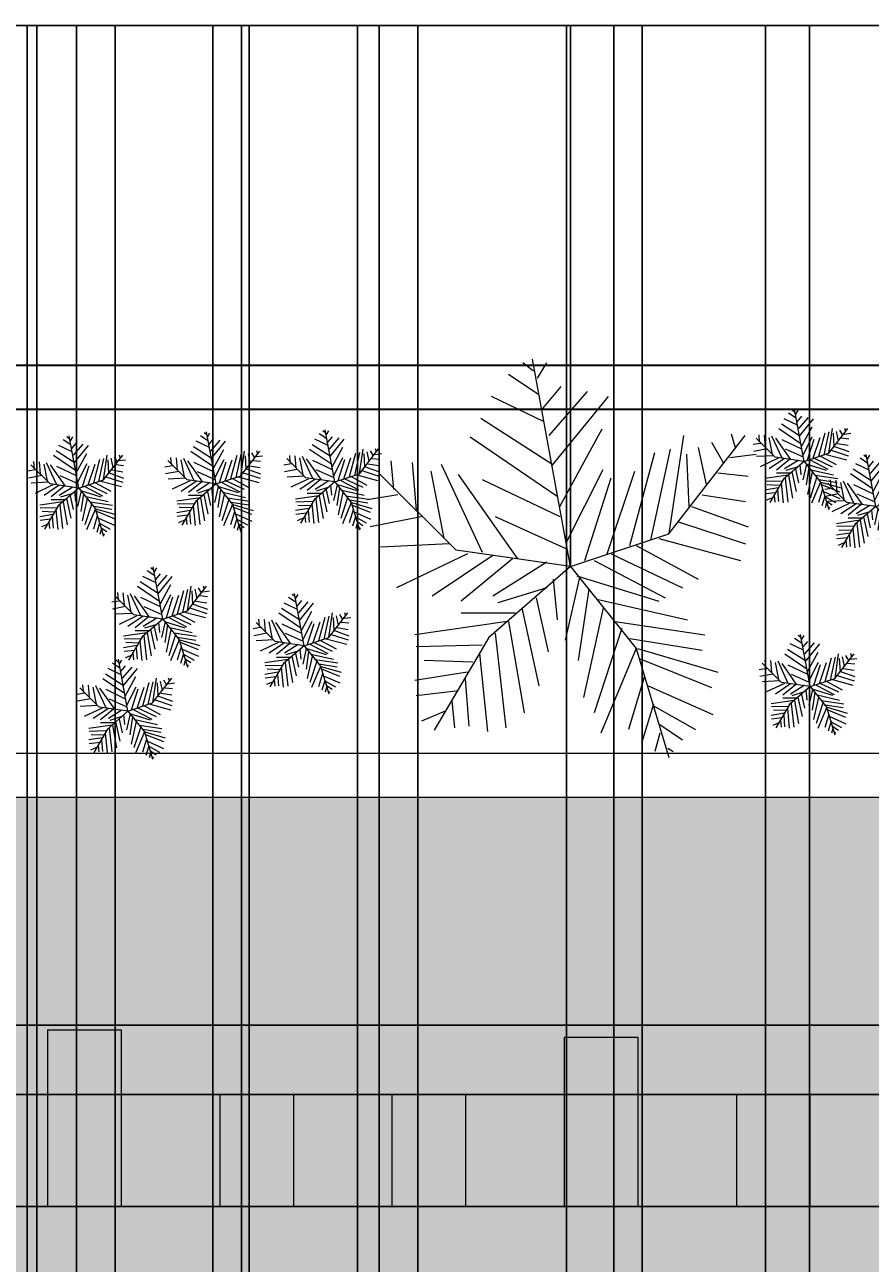
# Model space of a CAD drawing. Units: inches. Extents: x 818 to 1898, y 976 to 2364.
# Tile 94 of 96: x 1439 to 1612, y 2111 to 2364. Entities that reach past the tile are written whole.
import ezdxf

# ---------------------------------------------------------------- set-up
doc = ezdxf.new("R2010")
doc.units = ezdxf.units.IN
doc.header["$LTSCALE"] = 5
doc.header["$MEASUREMENT"] = 0
for name, color, linetype, lineweight in [('A-ANNO-DIMS', 2, 'Continuous', 18), ('C-PROP', 7, 'Continuous', 35), ('L-PAVE', 8, 'Continuous', 18), ('L-PLNT-BEDS', 94, 'Continuous', 18)]:
    doc.layers.add(name, color=color, linetype=linetype, lineweight=lineweight)
for name, color, linetype, lineweight, true_color in [('L-PAVE-PATT', 9, 'Continuous', 9, 0xc7c8ca), ('L-PLNT', 116, 'Continuous', 13, 0x136734), ('L-PLNT-PATT', 114, 'Continuous', 9, 0x139b48)]:
    doc.layers.add(name, color=color, linetype=linetype, lineweight=lineweight, true_color=true_color)
doc.styles.get("Standard").update_dxf_attribs({"font": 'arial.ttf'})
doc.dimstyles.get("Standard").update_dxf_attribs({"dimtxt": 0.18, "dimasz": 0.18, "dimexe": 0.18, "dimexo": 0.0625, "dimgap": 0.09, "dimtad": 0, "dimtih": 1, "dimtoh": 1, "dimdec": 4, "dimzin": 0, "dimdsep": 46, "dimtxsty": 'Standard', "dimcen": 0.09, "dimadec": 0, "dimazin": 0, "dimtfac": 1, "dimtdec": 4, "dimtofl": 0, "dimtmove": 0, "dimatfit": 3, "dimfxl": 1, "dimtolj": 1, "dimtzin": 0, "dimarcsym": 0})

# ---------------------------------------------------------------- blocks, each defined once
blk = doc.blocks.new('SHRUB-ACCENT')
for p, q in [((8.53, 19.84), (7.99, 20.28)), ((10.44, 9.82), (8.47, 20.47)), ((8.74, 19.5), (9.21, 20.28)), ((9.08, 17.24), (6.37, 18.54)), ((8.8, 18.63), (7.25, 19.67)), ((9.01, 17.93), (9.96, 19.06)), ((9.35, 16.54), (11.31, 18.8)), ((9.48, 14.98), (12.39, 18.54)), ((1.35, 13.77), (1.22, 15.24)), ((9.75, 13.42), (5.28, 16.46)), ((9.48, 15.07), (5.82, 17.41)), ((9.89, 12.9), (12.06, 16.89)), ((13.48, 10.9), (14.76, 15.68)), ((14.56, 11.16), (15.58, 15.85)), ((15.49, 11.5), (19.41, 16.55)), ((15.51, 11.51), (16.25, 16.54)), ((16.39, 15.59), (16.53, 12.9)), ((17, 15.94), (17.41, 14.03)), ((17.68, 16.2), (18.29, 15.16)), ((18.62, 15.42), (19.98, 15.59)), ((18.69, 16.63), (18.9, 15.94)), ((1.56, 13.51), (0, 13.25)), ((4.55, 10.66), (0.62, 14.58)), ((2.3, 15.16), (2.51, 12.72)), ((3.25, 14.72), (3.93, 11.25)), ((3.79, 15.07), (5.89, 10.55)), ((7.72, 10.21), (4.67, 14.55)), ((5.89, 14.29), (9.89, 12.38)), ((10.23, 11.07), (12.12, 14.81)), ((11.17, 10.12), (12.53, 14.37)), ((12.33, 10.47), (13.75, 14.72)), ((16.66, 12.9), (19.57, 11.86)), ((17.2, 13.51), (19.44, 13.16)), ((18.02, 14.63), (19.57, 14.46)), ((2.84, 12.38), (0.14, 11.86)), ((4.2, 10.99), (0.68, 10.81)), ((5.15, 10.47), (1.49, 8.73)), ((6.43, 10.38), (3.32, 8.3)), ((10.44, 9.82), (4.55, 10.66)), ((7.45, 10.21), (4.81, 8.04)), ((6.57, 12.38), (10.23, 10.73)), ((10.44, 9.82), (15.49, 11.5)), ((12.53, 10.47), (16.19, 8.73)), ((13.82, 10.9), (17, 9.16)), ((14.97, 11.25), (19.17, 10.12)), ((15.98, 12.12), (19.44, 10.99)), ((10.44, 9.82), (6.23, 6.17)), ((9.21, 10.03), (6.43, 8.3)), ((9.21, 8.73), (6.7, 7.95)), ((7.92, 7.69), (8.8, 3.69)), ((8.67, 8.21), (9.28, 5.43)), ((9.55, 9.16), (9.75, 7.08)), ((10.9, 9.25), (10.16, 6.04)), ((10.44, 9.82), (13.8, 5.61)), ((10.77, 9.34), (14.97, 8.04)), ((11.38, 8.64), (10.84, 5)), ((12.12, 7.69), (11.11, 3.09)), ((11.65, 10.12), (15.31, 8.21)), ((11.85, 8.12), (16.46, 7.08)), ((7.18, 6.99), (2.44, 6.3)), ((5.89, 5.78), (2.51, 5.69)), ((6.23, 6.17), (3.43, 1.4)), ((7.59, 7.43), (4.81, 7.43)), ((5.76, 5.34), (6.16, 1.35)), ((6.57, 6.39), (7.11, 1.52)), ((7.25, 6.99), (8.06, 2.31)), ((13.07, 6.65), (11.65, 2.31)), ((13.82, 5.6), (11.99, 1.26)), ((12.73, 6.99), (17.34, 6.3)), ((13.48, 6.13), (17.2, 5.52)), ((13.8, 5.61), (15.49, 0)), ((13.88, 5.6), (18.02, 4.39)), ((14.02, 5.08), (17.68, 3.61)), ((5.15, 4.39), (2.44, 3.95)), ((4.67, 3.43), (2.51, 3.17)), ((5.42, 4.91), (2.91, 5)), ((4.33, 2.91), (4.47, 1.52)), ((5.01, 4.04), (5.21, 1.61)), ((14.22, 4.13), (13.41, 1.44)), ((14.7, 2.74), (14.09, 0.74)), ((14.43, 3.69), (17.74, 2.22)), ((14.7, 2.65), (16.86, 1.44)), ((4, 2.39), (2.78, 1.87)), ((15.04, 1.26), (14.76, 0.31)), ((15.04, 1.7), (16.19, 0.92)), ((15.44, 0.48), (15.71, 0.31))]:
    blk.add_line(p, q)
blk = doc.blocks.new('PALM-BORDER')
for p, q in [((41.53, 39.05), (33.72, 81.45)), ((33.95, 78.95), (31.8, 80.68)), ((34.76, 77.57), (36.65, 80.68)), ((35.03, 74.11), (28.83, 78.26)), ((36.11, 68.59), (25.33, 73.77)), ((35.84, 71.35), (39.61, 75.84)), ((37.18, 65.82), (45, 74.8)), ((37.72, 59.6), (49.31, 73.77)), ((37.72, 59.95), (23.17, 69.28)), ((39.34, 51.31), (47.96, 67.2)), ((61.61, 45.75), (77.23, 65.83)), ((61.71, 45.79), (64.67, 65.82)), ((74.37, 66.17), (75.18, 63.4)), ((38.8, 53.39), (21.02, 65.48)), ((67.63, 63.4), (69.25, 55.81)), ((70.33, 64.44), (72.75, 60.3)), ((53.62, 43.37), (58.74, 62.37)), ((57.93, 44.41), (61.97, 63.06)), ((65.21, 62.02), (65.75, 51.31)), ((74.1, 61.33), (79.49, 62.02)), ((5.39, 54.77), (4.85, 60.64)), ((9.16, 60.3), (9.97, 50.62)), ((12.93, 58.57), (15.63, 44.75)), ((15.09, 59.95), (23.44, 41.99)), ((40.69, 44.06), (48.23, 58.91)), ((49.04, 41.64), (54.7, 58.57)), ((71.68, 58.22), (77.87, 57.53)), ((18.1, 42.4), (2.48, 58.02)), ((30.72, 40.61), (18.59, 57.88)), ((23.44, 56.84), (39.34, 49.24)), ((44.46, 40.26), (49.85, 57.19)), ((6.2, 53.73), (0, 52.7)), ((68.44, 53.73), (77.33, 52.35)), ((66.29, 51.31), (77.87, 47.17)), ((11.32, 49.24), (0.54, 47.17)), ((26.14, 49.24), (40.69, 42.68)), ((63.59, 48.21), (77.33, 43.71)), ((41.53, 39.05), (61.61, 45.75)), ((16.71, 43.71), (2.69, 43.02)), ((54.97, 43.37), (67.63, 36.46)), ((59.55, 44.75), (76.26, 40.26)), ((20.48, 41.64), (5.93, 34.73)), ((25.6, 41.3), (13.2, 33.01)), ((41.53, 39.05), (18.1, 42.4)), ((29.64, 40.61), (19.13, 31.97)), ((49.85, 41.64), (64.4, 34.73)), ((41.53, 39.05), (24.79, 24.55)), ((36.65, 39.91), (25.6, 33.01)), ((41.53, 39.05), (54.92, 22.32)), ((46.35, 40.26), (60.9, 32.66)), ((37.99, 36.46), (38.8, 28.17)), ((43.38, 36.81), (40.42, 24.02)), ((42.84, 37.15), (59.55, 31.97)), ((36.65, 34.73), (26.68, 31.62)), ((45.27, 34.39), (43.11, 19.88)), ((31.53, 30.59), (35.03, 14.7)), ((34.49, 32.66), (36.92, 21.61)), ((48.23, 30.59), (44.19, 12.28)), ((47.15, 32.32), (65.48, 28.17)), ((30.18, 29.55), (19.13, 29.55)), ((28.56, 27.82), (9.7, 25.06)), ((26.14, 25.41), (28.29, 6.06)), ((28.83, 27.82), (32.07, 9.17)), ((52, 26.44), (46.35, 9.17)), ((50.66, 27.82), (68.98, 25.06)), ((23.44, 22.99), (9.97, 22.64)), ((24.79, 24.55), (13.63, 5.58)), ((53.62, 24.37), (68.44, 21.95)), ((22.9, 21.26), (24.52, 5.37)), ((54.97, 22.3), (47.69, 5.02)), ((54.92, 22.32), (61.61, 0)), ((55.24, 22.3), (71.68, 17.46)), ((21.56, 19.53), (11.59, 19.88)), ((55.78, 20.22), (70.33, 14.35)), ((20.48, 17.46), (9.7, 15.73)), ((19.94, 16.08), (20.75, 6.41)), ((56.59, 16.42), (53.35, 5.72)), ((18.59, 13.66), (9.97, 12.62)), ((57.39, 14.7), (70.6, 8.83)), ((17.24, 11.59), (17.78, 6.06)), ((58.47, 10.9), (56.05, 2.95)), ((58.47, 10.55), (67.09, 5.72)), ((15.9, 9.52), (11.05, 7.44)), ((59.82, 6.75), (64.4, 3.64)), ((59.82, 5.02), (58.74, 1.22)), ((61.44, 1.92), (62.51, 1.22))]:
    blk.add_line(p, q)
blk = doc.blocks.new('*D57')
at = {"layer": 'A-ANNO-DIMS', "color": 0, "lineweight": -2, "ltscale": 5, "transparency": 16777216}
for p, q in [((992.73, 2294.28), (992.73, 2363.87)), ((992.91, 2363.69), (1395.43, 2363.69)), ((1798.54, 2363.69), (1396.01, 2363.69)), ((1798.72, 2294.28), (1798.72, 2363.87))]:
    blk.add_line(p, q, dxfattribs=at)
at = {"layer": 'A-ANNO-DIMS', "color": 0, "ltscale": 5, "transparency": 16777216}
for points in [[(992.91, 2363.72), (992.91, 2363.66), (992.73, 2363.69)], [(1798.54, 2363.72), (1798.54, 2363.66), (1798.72, 2363.69)]]:
    blk.add_solid(points, dxfattribs=at)
at = {"layer": 'Defpoints', "color": 0, "ltscale": 5, "transparency": 16777216}
for p in [(1798.72, 2363.69), (992.73, 2294.22), (1798.72, 2294.22)]:
    blk.add_point(p, dxfattribs=at)
at = {"layer": 'A-ANNO-DIMS', "color": 0, "ltscale": 5, "transparency": 16777216, "insert": (1395.72, 2363.69), "char_height": 0.18, "attachment_point": 5}
blk.add_mtext('\\A1;806', dxfattribs=at)
blk = doc.blocks.new('*D86')
at = {"layer": 'A-ANNO-DIMS', "color": 0, "lineweight": -2, "ltscale": 5, "transparency": 16777216}
for p, q in [((1258.73, 2053.14), (1258.73, 2363.87)), ((1258.91, 2363.69), (1486.43, 2363.69)), ((1714.55, 2363.69), (1487.02, 2363.69)), ((1714.73, 2053.14), (1714.73, 2363.87))]:
    blk.add_line(p, q, dxfattribs=at)
at = {"layer": 'A-ANNO-DIMS', "color": 0, "ltscale": 5, "transparency": 16777216}
for points in [[(1258.91, 2363.72), (1258.91, 2363.66), (1258.73, 2363.69)], [(1714.55, 2363.72), (1714.55, 2363.66), (1714.73, 2363.69)]]:
    blk.add_solid(points, dxfattribs=at)
at = {"layer": 'Defpoints', "color": 0, "ltscale": 5, "transparency": 16777216}
for p in [(1714.73, 2363.69), (1258.73, 2053.08), (1714.73, 2053.08)]:
    blk.add_point(p, dxfattribs=at)
at = {"layer": 'A-ANNO-DIMS', "color": 0, "ltscale": 5, "transparency": 16777216, "insert": (1486.73, 2363.69), "char_height": 0.18, "attachment_point": 5}
blk.add_mtext('\\A1;456', dxfattribs=at)
blk = doc.blocks.new('*D99')
at = {"layer": 'A-ANNO-DIMS', "color": 0, "lineweight": -2, "ltscale": 5, "transparency": 16777216}
for p, q in [((1391.88, 1071.12), (1391.88, 2363.87)), ((1392.06, 2363.69), (1420.45, 2363.69)), ((1449.64, 2363.69), (1421.24, 2363.69)), ((1449.82, 1071.12), (1449.82, 2363.87))]:
    blk.add_line(p, q, dxfattribs=at)
at = {"layer": 'A-ANNO-DIMS', "color": 0, "ltscale": 5, "transparency": 16777216}
for points in [[(1392.06, 2363.72), (1392.06, 2363.66), (1391.88, 2363.69)], [(1449.64, 2363.72), (1449.64, 2363.66), (1449.82, 2363.69)]]:
    blk.add_solid(points, dxfattribs=at)
at = {"layer": 'Defpoints', "color": 0, "ltscale": 5, "transparency": 16777216}
for p in [(1449.82, 2363.69), (1391.88, 1071.06), (1449.82, 1071.06)]:
    blk.add_point(p, dxfattribs=at)
at = {"layer": 'A-ANNO-DIMS', "color": 0, "ltscale": 5, "transparency": 16777216, "insert": (1420.85, 2363.69), "char_height": 0.18, "attachment_point": 5}
blk.add_mtext('\\A1;57.94', dxfattribs=at)
blk = doc.blocks.new('*D100')
at = {"layer": 'A-ANNO-DIMS', "color": 0, "lineweight": -2, "ltscale": 5, "transparency": 16777216}
for p, q in [((1449.82, 1071.12), (1449.82, 2363.87)), ((1450, 2363.69), (1478.17, 2363.69)), ((1507.12, 2363.69), (1478.95, 2363.69)), ((1507.3, 1071.12), (1507.3, 2363.87))]:
    blk.add_line(p, q, dxfattribs=at)
at = {"layer": 'A-ANNO-DIMS', "color": 0, "ltscale": 5, "transparency": 16777216}
for points in [[(1450, 2363.72), (1450, 2363.66), (1449.82, 2363.69)], [(1507.12, 2363.72), (1507.12, 2363.66), (1507.3, 2363.69)]]:
    blk.add_solid(points, dxfattribs=at)
at = {"layer": 'Defpoints', "color": 0, "ltscale": 5, "transparency": 16777216}
for p in [(1507.3, 2363.69), (1449.82, 1071.06), (1507.3, 1071.06)]:
    blk.add_point(p, dxfattribs=at)
at = {"layer": 'A-ANNO-DIMS', "color": 0, "ltscale": 5, "transparency": 16777216, "insert": (1478.56, 2363.69), "char_height": 0.18, "attachment_point": 5}
blk.add_mtext('\\A1;57.48', dxfattribs=at)
blk = doc.blocks.new('*D101')
at = {"layer": 'A-ANNO-DIMS', "color": 0, "lineweight": -2, "ltscale": 5, "transparency": 16777216}
for p, q in [((1507.3, 1071.12), (1507.3, 2363.87)), ((1507.48, 2363.69), (1536, 2363.69)), ((1565.3, 2363.69), (1536.78, 2363.69)), ((1565.48, 1071.12), (1565.48, 2363.87))]:
    blk.add_line(p, q, dxfattribs=at)
at = {"layer": 'A-ANNO-DIMS', "color": 0, "ltscale": 5, "transparency": 16777216}
for points in [[(1507.48, 2363.72), (1507.48, 2363.66), (1507.3, 2363.69)], [(1565.3, 2363.72), (1565.3, 2363.66), (1565.48, 2363.69)]]:
    blk.add_solid(points, dxfattribs=at)
at = {"layer": 'Defpoints', "color": 0, "ltscale": 5, "transparency": 16777216}
for p in [(1565.48, 2363.69), (1507.3, 1071.06), (1565.48, 1071.06)]:
    blk.add_point(p, dxfattribs=at)
at = {"layer": 'A-ANNO-DIMS', "color": 0, "ltscale": 5, "transparency": 16777216, "insert": (1536.39, 2363.69), "char_height": 0.18, "attachment_point": 5}
blk.add_mtext('\\A1;58.19', dxfattribs=at)
blk = doc.blocks.new('*D102')
at = {"layer": 'A-ANNO-DIMS', "color": 0, "lineweight": -2, "ltscale": 5, "transparency": 16777216}
for p, q in [((1565.48, 1071.12), (1565.48, 2363.87)), ((1565.66, 2363.69), (1595.63, 2363.69)), ((1626.39, 2363.69), (1596.42, 2363.69)), ((1626.57, 1071.12), (1626.57, 2363.87))]:
    blk.add_line(p, q, dxfattribs=at)
at = {"layer": 'A-ANNO-DIMS', "color": 0, "ltscale": 5, "transparency": 16777216}
for points in [[(1565.66, 2363.72), (1565.66, 2363.66), (1565.48, 2363.69)], [(1626.39, 2363.72), (1626.39, 2363.66), (1626.57, 2363.69)]]:
    blk.add_solid(points, dxfattribs=at)
at = {"layer": 'Defpoints', "color": 0, "ltscale": 5, "transparency": 16777216}
for p in [(1626.57, 2363.69), (1565.48, 1071.06), (1626.57, 1071.06)]:
    blk.add_point(p, dxfattribs=at)
at = {"layer": 'A-ANNO-DIMS', "color": 0, "ltscale": 5, "transparency": 16777216, "insert": (1596.03, 2363.69), "char_height": 0.18, "attachment_point": 5}
blk.add_mtext('\\A1;61.09', dxfattribs=at)
blk = doc.blocks.new('*D138')
at = {"layer": 'A-ANNO-DIMS', "color": 0, "lineweight": -2, "ltscale": 5, "transparency": 16777216}
for p, q in [((1400.78, 2245.03), (1400.78, 2363.87)), ((1400.96, 2363.69), (1475.45, 2363.69)), ((1550.69, 2363.69), (1476.19, 2363.69)), ((1550.87, 2253.22), (1550.87, 2363.87))]:
    blk.add_line(p, q, dxfattribs=at)
at = {"layer": 'A-ANNO-DIMS', "color": 0, "ltscale": 5, "transparency": 16777216}
for points in [[(1400.96, 2363.72), (1400.96, 2363.66), (1400.78, 2363.69)], [(1550.69, 2363.72), (1550.69, 2363.66), (1550.87, 2363.69)]]:
    blk.add_solid(points, dxfattribs=at)
at = {"layer": 'Defpoints', "color": 0, "ltscale": 5, "transparency": 16777216}
for p in [(1550.87, 2363.69), (1550.87, 2253.16), (1400.78, 2244.97)]:
    blk.add_point(p, dxfattribs=at)
at = {"layer": 'A-ANNO-DIMS', "color": 0, "ltscale": 5, "transparency": 16777216, "insert": (1475.82, 2363.69), "char_height": 0.18, "attachment_point": 5}
blk.add_mtext('\\A1;150.1', dxfattribs=at)
blk = doc.blocks.new('*D139')
at = {"layer": 'A-ANNO-DIMS', "color": 0, "lineweight": -2, "ltscale": 5, "transparency": 16777216}
for p, q in [((1550.87, 2253.22), (1550.87, 2363.87)), ((1551.05, 2363.69), (1629.62, 2363.69)), ((1708.97, 2363.69), (1630.39, 2363.69)), ((1709.15, 2245.03), (1709.15, 2363.87))]:
    blk.add_line(p, q, dxfattribs=at)
at = {"layer": 'A-ANNO-DIMS', "color": 0, "ltscale": 5, "transparency": 16777216}
for points in [[(1551.05, 2363.72), (1551.05, 2363.66), (1550.87, 2363.69)], [(1708.97, 2363.72), (1708.97, 2363.66), (1709.15, 2363.69)]]:
    blk.add_solid(points, dxfattribs=at)
at = {"layer": 'Defpoints', "color": 0, "ltscale": 5, "transparency": 16777216}
for p in [(1709.15, 2363.69), (1550.87, 2253.16), (1709.15, 2244.97)]:
    blk.add_point(p, dxfattribs=at)
at = {"layer": 'A-ANNO-DIMS', "color": 0, "ltscale": 5, "transparency": 16777216, "insert": (1630.01, 2363.69), "char_height": 0.18, "attachment_point": 5}
blk.add_mtext('\\A1;158.3', dxfattribs=at)
blk = doc.blocks.new('*D147')
at = {"layer": 'A-ANNO-DIMS', "color": 0, "lineweight": -2, "ltscale": 5, "transparency": 16777216}
for p, q in [((1212.58, 2145.25), (1897.92, 2145.25)), ((1897.74, 2145.07), (1897.74, 2133.99)), ((1897.74, 2122.56), (1897.74, 2133.63)), ((1212.58, 2122.38), (1897.92, 2122.38))]:
    blk.add_line(p, q, dxfattribs=at)
at = {"layer": 'A-ANNO-DIMS', "color": 0, "ltscale": 5, "transparency": 16777216}
for points in [[(1897.71, 2145.07), (1897.77, 2145.07), (1897.74, 2145.25)], [(1897.71, 2122.56), (1897.77, 2122.56), (1897.74, 2122.38)]]:
    blk.add_solid(points, dxfattribs=at)
at = {"layer": 'Defpoints', "color": 0, "ltscale": 5, "transparency": 16777216}
for p in [(1212.52, 2145.25), (1897.74, 2145.25), (1212.52, 2122.38)]:
    blk.add_point(p, dxfattribs=at)
at = {"layer": 'A-ANNO-DIMS', "color": 0, "ltscale": 5, "transparency": 16777216, "insert": (1897.74, 2133.81), "char_height": 0.18, "attachment_point": 5}
blk.add_mtext('\\A1;22.87', dxfattribs=at)
blk = doc.blocks.new('*D148')
at = {"layer": 'A-ANNO-DIMS', "color": 0, "lineweight": -2, "ltscale": 5, "transparency": 16777216}
for p, q in [((1232.67, 2159.43), (1897.92, 2159.43)), ((1897.74, 2159.25), (1897.74, 2141.09)), ((1897.74, 2122.56), (1897.74, 2140.72)), ((1232.67, 2122.38), (1897.92, 2122.38))]:
    blk.add_line(p, q, dxfattribs=at)
at = {"layer": 'A-ANNO-DIMS', "color": 0, "ltscale": 5, "transparency": 16777216}
for points in [[(1897.71, 2159.25), (1897.77, 2159.25), (1897.74, 2159.43)], [(1897.71, 2122.56), (1897.77, 2122.56), (1897.74, 2122.38)]]:
    blk.add_solid(points, dxfattribs=at)
at = {"layer": 'Defpoints', "color": 0, "ltscale": 5, "transparency": 16777216}
for p in [(1232.61, 2159.43), (1897.74, 2159.43), (1232.61, 2122.38)]:
    blk.add_point(p, dxfattribs=at)
at = {"layer": 'A-ANNO-DIMS', "color": 0, "ltscale": 5, "transparency": 16777216, "insert": (1897.74, 2140.9), "char_height": 0.18, "attachment_point": 5}
blk.add_mtext('\\A1;37.05', dxfattribs=at)
blk = doc.blocks.new('*D161')
at = {"layer": 'A-ANNO-DIMS', "color": 0, "lineweight": -2, "ltscale": 5, "transparency": 16777216}
for p, q in [((1429.23, 1876.14), (1429.23, 2363.87)), ((1429.41, 2363.69), (1509.59, 2363.69)), ((1590.55, 2363.69), (1510.36, 2363.69)), ((1590.73, 1876.14), (1590.73, 2363.87))]:
    blk.add_line(p, q, dxfattribs=at)
at = {"layer": 'A-ANNO-DIMS', "color": 0, "ltscale": 5, "transparency": 16777216}
for points in [[(1429.41, 2363.72), (1429.41, 2363.66), (1429.23, 2363.69)], [(1590.55, 2363.72), (1590.55, 2363.66), (1590.73, 2363.69)]]:
    blk.add_solid(points, dxfattribs=at)
at = {"layer": 'Defpoints', "color": 0, "ltscale": 5, "transparency": 16777216}
for p in [(1590.73, 2363.69), (1429.23, 1876.08), (1590.73, 1876.08)]:
    blk.add_point(p, dxfattribs=at)
at = {"layer": 'A-ANNO-DIMS', "color": 0, "ltscale": 5, "transparency": 16777216, "insert": (1509.98, 2363.69), "char_height": 0.18, "attachment_point": 5}
blk.add_mtext('\\A1;161.5', dxfattribs=at)
blk = doc.blocks.new('*D169')
at = {"layer": 'A-ANNO-DIMS', "color": 0, "lineweight": -2, "ltscale": 5, "transparency": 16777216}
for p, q in [((1441.73, 1600.14), (1441.73, 2363.87)), ((1441.91, 2363.69), (1459.51, 2363.69)), ((1477.55, 2363.69), (1459.94, 2363.69)), ((1477.73, 1600.14), (1477.73, 2363.87))]:
    blk.add_line(p, q, dxfattribs=at)
at = {"layer": 'A-ANNO-DIMS', "color": 0, "ltscale": 5, "transparency": 16777216}
for points in [[(1441.91, 2363.72), (1441.91, 2363.66), (1441.73, 2363.69)], [(1477.55, 2363.72), (1477.55, 2363.66), (1477.73, 2363.69)]]:
    blk.add_solid(points, dxfattribs=at)
at = {"layer": 'Defpoints', "color": 0, "ltscale": 5, "transparency": 16777216}
for p in [(1477.73, 2363.69), (1441.73, 1600.08), (1477.73, 1600.08)]:
    blk.add_point(p, dxfattribs=at)
at = {"layer": 'A-ANNO-DIMS', "color": 0, "ltscale": 5, "transparency": 16777216, "insert": (1459.73, 2363.69), "char_height": 0.18, "attachment_point": 5}
blk.add_mtext('\\A1;36', dxfattribs=at)
blk = doc.blocks.new('*D175')
at = {"layer": 'A-ANNO-DIMS', "color": 0, "lineweight": -2, "ltscale": 5, "transparency": 16777216}
for p, q in [((1559.73, 1647.64), (1559.73, 2363.87)), ((1559.91, 2363.69), (1614.45, 2363.69)), ((1669.55, 2363.69), (1615.01, 2363.69)), ((1669.73, 1647.64), (1669.73, 2363.87))]:
    blk.add_line(p, q, dxfattribs=at)
at = {"layer": 'A-ANNO-DIMS', "color": 0, "ltscale": 5, "transparency": 16777216}
for points in [[(1559.91, 2363.72), (1559.91, 2363.66), (1559.73, 2363.69)], [(1669.55, 2363.72), (1669.55, 2363.66), (1669.73, 2363.69)]]:
    blk.add_solid(points, dxfattribs=at)
at = {"layer": 'Defpoints', "color": 0, "ltscale": 5, "transparency": 16777216}
for p in [(1669.73, 2363.69), (1559.73, 1647.58), (1669.73, 1647.58)]:
    blk.add_point(p, dxfattribs=at)
at = {"layer": 'A-ANNO-DIMS', "color": 0, "ltscale": 5, "transparency": 16777216, "insert": (1614.73, 2363.69), "char_height": 0.18, "attachment_point": 5}
blk.add_mtext('\\A1;110', dxfattribs=at)
blk = doc.blocks.new('*D196')
at = {"layer": 'A-ANNO-DIMS', "color": 0, "lineweight": -2, "ltscale": 5, "transparency": 16777216}
for p, q in [((1439.73, 1526.73), (1439.73, 2363.87)), ((1439.91, 2363.69), (1448.51, 2363.69)), ((1457.55, 2363.69), (1448.94, 2363.69)), ((1457.73, 1526.73), (1457.73, 2363.87))]:
    blk.add_line(p, q, dxfattribs=at)
at = {"layer": 'A-ANNO-DIMS', "color": 0, "ltscale": 5, "transparency": 16777216}
for points in [[(1439.91, 2363.72), (1439.91, 2363.66), (1439.73, 2363.69)], [(1457.55, 2363.72), (1457.55, 2363.66), (1457.73, 2363.69)]]:
    blk.add_solid(points, dxfattribs=at)
at = {"layer": 'Defpoints', "color": 0, "ltscale": 5, "transparency": 16777216}
for p in [(1457.73, 2363.69), (1439.73, 1526.67), (1457.73, 1526.67)]:
    blk.add_point(p, dxfattribs=at)
at = {"layer": 'A-ANNO-DIMS', "color": 0, "ltscale": 5, "transparency": 16777216, "insert": (1448.73, 2363.69), "char_height": 0.18, "attachment_point": 5}
blk.add_mtext('\\A1;18', dxfattribs=at)
blk = doc.blocks.new('*D203')
at = {"layer": 'A-ANNO-DIMS', "color": 0, "lineweight": -2, "ltscale": 5, "transparency": 16777216}
for p, q in [((1599.73, 1876.14), (1599.73, 2363.87)), ((1599.91, 2363.69), (1652.44, 2363.69)), ((1705.55, 2363.69), (1653.01, 2363.69)), ((1705.73, 1876.14), (1705.73, 2363.87))]:
    blk.add_line(p, q, dxfattribs=at)
at = {"layer": 'A-ANNO-DIMS', "color": 0, "ltscale": 5, "transparency": 16777216}
for points in [[(1599.91, 2363.72), (1599.91, 2363.66), (1599.73, 2363.69)], [(1705.55, 2363.72), (1705.55, 2363.66), (1705.73, 2363.69)]]:
    blk.add_solid(points, dxfattribs=at)
at = {"layer": 'Defpoints', "color": 0, "ltscale": 5, "transparency": 16777216}
for p in [(1705.73, 2363.69), (1599.73, 1876.08), (1705.73, 1876.08)]:
    blk.add_point(p, dxfattribs=at)
at = {"layer": 'A-ANNO-DIMS', "color": 0, "ltscale": 5, "transparency": 16777216, "insert": (1652.73, 2363.69), "char_height": 0.18, "attachment_point": 5}
blk.add_mtext('\\A1;106', dxfattribs=at)
blk = doc.blocks.new('*D205')
at = {"layer": 'A-ANNO-DIMS', "color": 0, "lineweight": -2, "ltscale": 5, "transparency": 16777216}
for p, q in [((1590.73, 2044.14), (1590.73, 2363.87)), ((1590.91, 2363.69), (1652.45, 2363.69)), ((1714.55, 2363.69), (1653.01, 2363.69)), ((1714.73, 2053.14), (1714.73, 2363.87))]:
    blk.add_line(p, q, dxfattribs=at)
at = {"layer": 'A-ANNO-DIMS', "color": 0, "ltscale": 5, "transparency": 16777216}
for points in [[(1590.91, 2363.72), (1590.91, 2363.66), (1590.73, 2363.69)], [(1714.55, 2363.72), (1714.55, 2363.66), (1714.73, 2363.69)]]:
    blk.add_solid(points, dxfattribs=at)
at = {"layer": 'Defpoints', "color": 0, "ltscale": 5, "transparency": 16777216}
for p in [(1714.73, 2363.69), (1714.73, 2053.08), (1590.73, 2044.08)]:
    blk.add_point(p, dxfattribs=at)
at = {"layer": 'A-ANNO-DIMS', "color": 0, "ltscale": 5, "transparency": 16777216, "insert": (1652.73, 2363.69), "char_height": 0.18, "attachment_point": 5}
blk.add_mtext('\\A1;124', dxfattribs=at)
blk = doc.blocks.new('*D238')
at = {"layer": 'A-ANNO-DIMS', "color": 0, "lineweight": -2, "ltscale": 5, "transparency": 16777216}
for p, q in [((1483.55, 1948.72), (1483.55, 2363.87)), ((1483.73, 2363.69), (1516.38, 2363.69)), ((1549.83, 2363.69), (1517.17, 2363.69)), ((1550.01, 1948.72), (1550.01, 2363.87))]:
    blk.add_line(p, q, dxfattribs=at)
at = {"layer": 'A-ANNO-DIMS', "color": 0, "ltscale": 5, "transparency": 16777216}
for points in [[(1483.73, 2363.72), (1483.73, 2363.66), (1483.55, 2363.69)], [(1549.83, 2363.72), (1549.83, 2363.66), (1550.01, 2363.69)]]:
    blk.add_solid(points, dxfattribs=at)
at = {"layer": 'Defpoints', "color": 0, "ltscale": 5, "transparency": 16777216}
for p in [(1550.01, 2363.69), (1483.55, 1948.66), (1550.01, 1948.66)]:
    blk.add_point(p, dxfattribs=at)
at = {"layer": 'A-ANNO-DIMS', "color": 0, "ltscale": 5, "transparency": 16777216, "insert": (1516.78, 2363.69), "char_height": 0.18, "attachment_point": 5}
blk.add_mtext('\\A1;66.47', dxfattribs=at)
blk = doc.blocks.new('*D240')
at = {"layer": 'A-ANNO-DIMS', "color": 0, "lineweight": -2, "ltscale": 5, "transparency": 16777216}
for p, q in [((1550.01, 1979.31), (1550.01, 2363.87)), ((1550.19, 2363.69), (1569.9, 2363.69)), ((1590.55, 2363.69), (1570.83, 2363.69)), ((1590.73, 1981.14), (1590.73, 2363.87))]:
    blk.add_line(p, q, dxfattribs=at)
at = {"layer": 'A-ANNO-DIMS', "color": 0, "ltscale": 5, "transparency": 16777216}
for points in [[(1550.19, 2363.72), (1550.19, 2363.66), (1550.01, 2363.69)], [(1590.55, 2363.72), (1590.55, 2363.66), (1590.73, 2363.69)]]:
    blk.add_solid(points, dxfattribs=at)
at = {"layer": 'Defpoints', "color": 0, "ltscale": 5, "transparency": 16777216}
for p in [(1590.73, 2363.69), (1550.01, 1979.24), (1590.73, 1981.08)]:
    blk.add_point(p, dxfattribs=at)
at = {"layer": 'A-ANNO-DIMS', "color": 0, "ltscale": 5, "transparency": 16777216, "insert": (1570.37, 2363.69), "char_height": 0.18, "attachment_point": 5}
blk.add_mtext('\\A1;40.714', dxfattribs=at)
blk = doc.blocks.new('*D244')
at = {"layer": 'A-ANNO-DIMS', "color": 0, "lineweight": -2, "ltscale": 5, "transparency": 16777216}
for p, q in [((1519.64, 1900.14), (1519.64, 2363.87)), ((1519.82, 2363.69), (1554.79, 2363.69)), ((1590.55, 2363.69), (1555.58, 2363.69)), ((1590.73, 1900.14), (1590.73, 2363.87))]:
    blk.add_line(p, q, dxfattribs=at)
at = {"layer": 'A-ANNO-DIMS', "color": 0, "ltscale": 5, "transparency": 16777216}
for points in [[(1519.82, 2363.72), (1519.82, 2363.66), (1519.64, 2363.69)], [(1590.55, 2363.72), (1590.55, 2363.66), (1590.73, 2363.69)]]:
    blk.add_solid(points, dxfattribs=at)
at = {"layer": 'Defpoints', "color": 0, "ltscale": 5, "transparency": 16777216}
for p in [(1590.73, 2363.69), (1519.64, 1900.08), (1590.73, 1900.08)]:
    blk.add_point(p, dxfattribs=at)
at = {"layer": 'A-ANNO-DIMS', "color": 0, "ltscale": 5, "transparency": 16777216, "insert": (1555.18, 2363.69), "char_height": 0.18, "attachment_point": 5}
blk.add_mtext('\\A1;71.08', dxfattribs=at)
blk = doc.blocks.new('*D258')
at = {"layer": 'A-ANNO-DIMS', "color": 0, "lineweight": -2, "ltscale": 5, "transparency": 16777216}
for p, q in [((1422.02, 2053.14), (1422.02, 2363.87)), ((1422.2, 2363.69), (1453.26, 2363.69)), ((1484.94, 2363.69), (1453.88, 2363.69)), ((1485.12, 2053.14), (1485.12, 2363.87))]:
    blk.add_line(p, q, dxfattribs=at)
at = {"layer": 'A-ANNO-DIMS', "color": 0, "ltscale": 5, "transparency": 16777216}
for points in [[(1422.2, 2363.72), (1422.2, 2363.66), (1422.02, 2363.69)], [(1484.94, 2363.72), (1484.94, 2363.66), (1485.12, 2363.69)]]:
    blk.add_solid(points, dxfattribs=at)
at = {"layer": 'Defpoints', "color": 0, "ltscale": 5, "transparency": 16777216}
for p in [(1485.12, 2363.69), (1422.02, 2053.08), (1485.12, 2053.08)]:
    blk.add_point(p, dxfattribs=at)
at = {"layer": 'A-ANNO-DIMS', "color": 0, "ltscale": 5, "transparency": 16777216, "insert": (1453.57, 2363.69), "char_height": 0.18, "attachment_point": 5}
blk.add_mtext('\\A1;63.1', dxfattribs=at)
blk = doc.blocks.new('*D281')
at = {"layer": 'A-ANNO-DIMS', "color": 0, "lineweight": -2, "ltscale": 5, "transparency": 16777216}
for p, q in [((1250.3, 1913.7), (1250.3, 2363.87)), ((1250.48, 2363.69), (1420.12, 2363.69)), ((1590.55, 2363.69), (1420.91, 2363.69)), ((1590.73, 2011.14), (1590.73, 2363.87))]:
    blk.add_line(p, q, dxfattribs=at)
at = {"layer": 'A-ANNO-DIMS', "color": 0, "ltscale": 5, "transparency": 16777216}
for points in [[(1250.48, 2363.72), (1250.48, 2363.66), (1250.3, 2363.69)], [(1590.55, 2363.72), (1590.55, 2363.66), (1590.73, 2363.69)]]:
    blk.add_solid(points, dxfattribs=at)
at = {"layer": 'Defpoints', "color": 0, "ltscale": 5, "transparency": 16777216}
for p in [(1590.73, 2363.69), (1590.73, 2011.08), (1250.3, 1913.64)]:
    blk.add_point(p, dxfattribs=at)
at = {"layer": 'A-ANNO-DIMS', "color": 0, "ltscale": 5, "transparency": 16777216, "insert": (1420.51, 2363.69), "char_height": 0.18, "attachment_point": 5}
blk.add_mtext('\\A1;340.4', dxfattribs=at)
blk = doc.blocks.new('*D288')
at = {"layer": 'A-ANNO-DIMS', "color": 0, "lineweight": -2, "ltscale": 5, "transparency": 16777216}
for p, q in [((1422.88, 1742.67), (1422.88, 2363.87)), ((1423.06, 2363.69), (1466.91, 2363.69)), ((1511.55, 2363.69), (1467.69, 2363.69)), ((1511.73, 1716.11), (1511.73, 2363.87))]:
    blk.add_line(p, q, dxfattribs=at)
at = {"layer": 'A-ANNO-DIMS', "color": 0, "ltscale": 5, "transparency": 16777216}
for points in [[(1423.06, 2363.72), (1423.06, 2363.66), (1422.88, 2363.69)], [(1511.55, 2363.72), (1511.55, 2363.66), (1511.73, 2363.69)]]:
    blk.add_solid(points, dxfattribs=at)
at = {"layer": 'Defpoints', "color": 0, "ltscale": 5, "transparency": 16777216}
for p in [(1511.73, 2363.69), (1422.88, 1742.61), (1511.73, 1716.05)]:
    blk.add_point(p, dxfattribs=at)
at = {"layer": 'A-ANNO-DIMS', "color": 0, "ltscale": 5, "transparency": 16777216, "insert": (1467.3, 2363.69), "char_height": 0.18, "attachment_point": 5}
blk.add_mtext('\\A1;88.85', dxfattribs=at)

msp = doc.modelspace()

# ---------------------------------------------------------------- hatches: boundary and pattern name
at = {"layer": 'L-PAVE-PATT', "ltscale": 5}
h = msp.add_hatch(color=256, dxfattribs=at)
h.dxf.hatch_style = 1
h.paths.add_polyline_path([(1212.5206, 2145.2461), (1197.3925, 2145.2461), (1197.3925, 2122.3767), (1212.5206, 2122.3767)])
h.paths.add_polyline_path([(1247.7373, 2159.4296), (1232.6091, 2159.4296), (1232.6091, 2122.3767), (1247.7373, 2122.3767)])
h.paths.add_polyline_path([(1282.9539, 2145.2461), (1267.8258, 2145.2461), (1267.8258, 2122.3767), (1282.9539, 2122.3767)])
h.paths.add_polyline_path([(1318.1705, 2145.2461), (1303.0424, 2145.2461), (1303.0424, 2122.3767), (1318.1705, 2122.3767)])
h.paths.add_polyline_path([(1353.3871, 2155.7839), (1338.259, 2155.7839), (1338.259, 2122.3767), (1353.3871, 2122.3767)])
h.paths.add_polyline_path([(1388.6037, 2145.2461), (1373.4756, 2145.2461), (1373.4756, 2122.3767), (1388.6037, 2122.3767)])
h.paths.add_polyline_path([(1423.8203, 2145.2461), (1408.6922, 2145.2461), (1408.6922, 2122.3767), (1423.8203, 2122.3767)])
h.paths.add_polyline_path([(1459.037, 2158.4222), (1443.9089, 2158.4222), (1443.9089, 2122.3767), (1459.037, 2122.3767)])
h.paths.add_polyline_path([(1494.2536, 2145.2461), (1479.1255, 2145.2461), (1479.1255, 2122.3767), (1494.2536, 2122.3767)])
h.paths.add_polyline_path([(1529.4702, 2145.2461), (1514.3421, 2145.2461), (1514.3421, 2122.3767), (1529.4702, 2122.3767)])
h.paths.add_polyline_path([(1564.6868, 2156.9246), (1549.5587, 2156.9246), (1549.5587, 2122.3767), (1564.6868, 2122.3767)])
h.paths.add_polyline_path([(1599.9034, 2145.2461), (1584.7753, 2145.2461), (1584.7753, 2122.3767), (1599.9034, 2122.3767)])
h.paths.add_polyline_path([(1635.1201, 2145.2461), (1619.9919, 2145.2461), (1619.9919, 2122.3767), (1635.1201, 2122.3767)])
h.paths.add_polyline_path([(1670.3367, 2156.1761), (1655.2086, 2156.1761), (1655.2086, 2122.3767), (1670.3367, 2122.3767)])
h.paths.add_polyline_path([(1701.7273, 2145.2461), (1686.5992, 2145.2461), (1686.5992, 2122.3767), (1701.7273, 2122.3767)])
h.paths.add_polyline_path([(1730.8897, 2145.2461), (1715.7616, 2145.2461), (1715.7616, 2122.3767), (1730.8897, 2122.3767)])
h.paths.add_polyline_path([(1776.3312, 2145.2461), (1753.1652, 2145.2461), (1753.1652, 2115.6891), (1776.3312, 2115.6891)])
at = {"layer": 'L-PLNT-PATT', "ltscale": 5}
h = msp.add_hatch(color=256, dxfattribs=at)
h.dxf.hatch_style = 1
h.paths.add_polyline_path([(1789.7173, 2205.9709), (1083.7252, 2205.9709), (1083.7252, 2083.2623), (1218.1114, 2083.2623), (1218.1114, 2053.0782), (1390.6356, 2053.0782), (1390.6356, 2081.1881), (1399.6356, 2081.1881), (1413.02, 2081.1881), (1422.02, 2081.1881), (1422.02, 2053.0782), (1676.6446, 2053.0782), (1676.6446, 2081.1881), (1714.7251, 2081.1881), (1714.7251, 2081.6235), (1789.7173, 2081.6235)])
h.paths.add_polyline_path([(1388.6037, 2145.2461), (1388.6037, 2122.3767), (1373.4756, 2122.3767), (1373.4756, 2145.2461)], flags=16)
h.paths.add_polyline_path([(1408.6922, 2145.2461), (1423.8203, 2145.2461), (1423.8203, 2122.3767), (1408.6922, 2122.3767)], flags=16)
h.paths.add_polyline_path([(1353.3871, 2155.7839), (1353.3871, 2122.3767), (1338.259, 2122.3767), (1338.259, 2155.7839)], flags=16)
h.paths.add_polyline_path([(1443.9089, 2158.4222), (1459.037, 2158.4222), (1459.037, 2122.3767), (1443.9089, 2122.3767)], flags=16)
h.paths.add_polyline_path([(1318.1705, 2145.2461), (1318.1705, 2122.3767), (1303.0424, 2122.3767), (1303.0424, 2145.2461)], flags=16)
h.paths.add_polyline_path([(1479.1255, 2145.2461), (1494.2536, 2145.2461), (1494.2536, 2122.3767), (1479.1255, 2122.3767)], flags=16)
h.paths.add_polyline_path([(1282.9539, 2145.2461), (1282.9539, 2122.3767), (1267.8258, 2122.3767), (1267.8258, 2145.2461)], flags=16)
h.paths.add_polyline_path([(1514.3421, 2145.2461), (1529.4702, 2145.2461), (1529.4702, 2122.3767), (1514.3421, 2122.3767)], flags=16)
h.paths.add_polyline_path([(1247.7373, 2159.4296), (1247.7373, 2122.3767), (1232.6091, 2122.3767), (1232.6091, 2159.4296)], flags=16)
h.paths.add_polyline_path([(1549.5587, 2156.9246), (1564.6868, 2156.9246), (1564.6868, 2122.3767), (1549.5587, 2122.3767)], flags=16)
h.paths.add_polyline_path([(1212.5206, 2145.2461), (1212.5206, 2122.3767), (1197.3925, 2122.3767), (1197.3925, 2145.2461)], flags=16)
h.paths.add_polyline_path([(1584.7753, 2145.2461), (1599.9034, 2145.2461), (1599.9034, 2122.3767), (1584.7753, 2122.3767)], flags=16)
h.paths.add_polyline_path([(1185.1073, 2104.7786), (1190.6407, 2104.7786), (1185.1073, 2098.2505), (1179.5738, 2104.7786)], flags=16)
h.paths.add_polyline_path([(1619.9919, 2145.2461), (1635.1201, 2145.2461), (1635.1201, 2122.3767), (1619.9919, 2122.3767)], flags=16)
h.paths.add_polyline_path([(1655.2086, 2156.1761), (1670.3367, 2156.1761), (1670.3367, 2122.3767), (1655.2086, 2122.3767)], flags=16)
h.paths.add_polyline_path([(1686.5992, 2145.2461), (1701.7273, 2145.2461), (1701.7273, 2122.3767), (1686.5992, 2122.3767)], flags=16)
h.paths.add_polyline_path([(1715.7616, 2145.2461), (1730.8897, 2145.2461), (1730.8897, 2122.3767), (1715.7616, 2122.3767)], flags=16)
h.paths.add_polyline_path([(1753.1652, 2145.2461), (1776.3312, 2145.2461), (1776.3312, 2115.6891), (1753.1652, 2115.6891)], flags=16)
h.paths.add_polyline_path([(1191.4331, 2146.5159), (1176.7891, 2146.5159), (1176.7891, 2134.1516), (1191.4331, 2134.1516)], flags=24)

# ---------------------------------------------------------------- linework, layer by layer
at = {"layer": 'C-PROP', "ltscale": 5}
for p, q in [((1798.7173, 2294.2171), (992.7251, 2294.2171)), ((1789.7173, 2285.2171), (1001.7252, 2285.2171))]:
    msp.add_line(p, q, dxfattribs=at)
at = {"layer": 'L-PAVE', "ltscale": 5}
for points in [[(1459.037, 2158.4222), (1443.9089, 2158.4222), (1443.9089, 2122.3767), (1459.037, 2122.3767)], [(1564.6868, 2156.9246), (1549.5587, 2156.9246), (1549.5587, 2122.3767), (1564.6868, 2122.3767)], [(1494.2536, 2145.2461), (1479.1255, 2145.2461), (1479.1255, 2122.3767), (1494.2536, 2122.3767)], [(1529.4702, 2145.2461), (1514.3421, 2145.2461), (1514.3421, 2122.3767), (1529.4702, 2122.3767)], [(1599.9034, 2145.2461), (1584.7753, 2145.2461), (1584.7753, 2122.3767), (1599.9034, 2122.3767)]]:
    msp.add_lwpolyline(points, close=True, dxfattribs=at)
at = {"layer": 'L-PLNT-BEDS', "ltscale": 5}
for p, q in [((1789.7173, 2214.9709), (1071.7252, 2214.9709)), ((1789.7173, 2205.9709), (1083.7252, 2205.9709))]:
    msp.add_line(p, q, dxfattribs=at)

# ---------------------------------------------------------------- block references
at = {"layer": 'L-PLNT'}
for name, p in [('PALM-BORDER', (1509.3373, 2214.1091)), ('SHRUB-ACCENT', (1588.1892, 2264.8219)), ('SHRUB-ACCENT', (1467.91, 2260.2161)), ('SHRUB-ACCENT', (1492.1974, 2260.6345)), ('SHRUB-ACCENT', (1439.8537, 2259.3793)), ('SHRUB-ACCENT', (1602.8454, 2255.617)), ('SHRUB-ACCENT', (1457.0225, 2232.6013)), ('SHRUB-ACCENT', (1485.9162, 2227.162)), ('SHRUB-ACCENT', (1589.4454, 2218.7972)), ('SHRUB-ACCENT', (1449.9037, 2213.773))]:
    msp.add_blockref(name, p, dxfattribs=at)

# ---------------------------------------------------------------- dimensions: what is measured, and where the dimension line sits
at = {"layer": 'A-ANNO-DIMS', "ltscale": 5}
for base, p1, p2, override, picture, middle in [((1798.7173, 2363.6929), (992.7251, 2294.2171), (1798.7173, 2294.2171), {"dimdec": 0, "dimlfac": 1, "dimrnd": 0, "dimzin": 0, "dimdsep": 46, "dimlunit": 2}, '*D57', (1395.7212, 2363.6929)), ((1590.7251, 2363.6929), (1250.3029, 1913.6401), (1590.7251, 2011.0782), {"dimdec": 1, "dimlfac": 1, "dimrnd": 0, "dimzin": 0, "dimdsep": 46, "dimlunit": 2}, '*D281', (1420.514, 2363.6929)), ((1714.7251, 2363.6929), (1258.7251, 2053.0782), (1714.7251, 2053.0782), {"dimdec": 0, "dimlfac": 1, "dimrnd": 0, "dimzin": 0, "dimdsep": 46, "dimlunit": 2}, '*D86', (1486.7251, 2363.6929)), ((1449.8196, 2363.6929), (1391.8757, 1071.0552), (1449.8196, 1071.0552), {"dimdec": 2, "dimlfac": 1, "dimrnd": 0, "dimzin": 0, "dimdsep": 46, "dimlunit": 2}, '*D99', (1420.8477, 2363.6929)), ((1550.8651, 2363.6929), (1400.7761, 2244.9688), (1550.8651, 2253.1602), {"dimdec": 1, "dimlfac": 1, "dimrnd": 0, "dimzin": 0, "dimdsep": 46, "dimlunit": 2}, '*D138', (1475.8206, 2363.6929)), ((1485.1216, 2363.6929), (1422.02, 2053.0782), (1485.1216, 2053.0782), {"dimdec": 1, "dimlfac": 1, "dimrnd": 0, "dimzin": 0, "dimdsep": 46, "dimlunit": 2}, '*D258', (1453.5708, 2363.6929)), ((1511.7251, 2363.6929), (1422.8756, 1742.6113), (1511.7251, 1716.0454), {"dimdec": 2, "dimlfac": 1, "dimrnd": 0, "dimzin": 0, "dimdsep": 46, "dimlunit": 2}, '*D288', (1467.3004, 2363.6929)), ((1590.7251, 2363.6929), (1429.2251, 1876.0782), (1590.7251, 1876.0782), {"dimdec": 1, "dimlfac": 1, "dimrnd": 0, "dimzin": 0, "dimdsep": 46, "dimlunit": 2}, '*D161', (1509.9751, 2363.6929)), ((1457.7251, 2363.6929), (1439.7251, 1526.6712), (1457.7251, 1526.6712), {"dimdec": 0, "dimlfac": 1, "dimrnd": 0, "dimzin": 0, "dimdsep": 46, "dimlunit": 2}, '*D196', (1448.7251, 2363.6929)), ((1477.7251, 2363.6929), (1441.7251, 1600.0782), (1477.7251, 1600.0782), {"dimdec": 0, "dimlfac": 1, "dimrnd": 0, "dimzin": 0, "dimdsep": 46, "dimlunit": 2}, '*D169', (1459.7251, 2363.6929)), ((1507.2982, 2363.6929), (1449.8196, 1071.0552), (1507.2982, 1071.0552), {"dimdec": 2, "dimlfac": 1, "dimrnd": 0, "dimzin": 0, "dimdsep": 46, "dimlunit": 2}, '*D100', (1478.5589, 2363.6929)), ((1550.0109, 2363.6929), (1483.5451, 1948.6602), (1550.0109, 1948.6602), {"dimdec": 2, "dimlfac": 1, "dimrnd": 0, "dimzin": 0, "dimdsep": 46, "dimlunit": 2}, '*D238', (1516.778, 2363.6929)), ((1565.4835, 2363.6929), (1507.2982, 1071.0552), (1565.4835, 1071.0552), {"dimdec": 2, "dimlfac": 1, "dimrnd": 0, "dimzin": 0, "dimdsep": 46, "dimlunit": 2}, '*D101', (1536.3908, 2363.6929)), ((1590.7251, 2363.6929), (1519.6413, 1900.0782), (1590.7251, 1900.0782), {"dimdec": 2, "dimlfac": 1, "dimrnd": 0, "dimzin": 0, "dimdsep": 46, "dimlunit": 2}, '*D244', (1555.1832, 2363.6929)), ((1590.7251, 2363.6929), (1550.0109, 1979.2444), (1590.7251, 1981.0782), {"dimdec": 3, "dimlfac": 1, "dimrnd": 0, "dimzin": 0, "dimdsep": 46, "dimlunit": 2}, '*D240', (1570.368, 2363.6929)), ((1709.1522, 2363.6929), (1550.8651, 2253.1602), (1709.1522, 2244.9688), {"dimdec": 1, "dimlfac": 1, "dimrnd": 0, "dimzin": 0, "dimdsep": 46, "dimlunit": 2}, '*D139', (1630.0087, 2363.6929)), ((1669.7251, 2363.6929), (1559.7251, 1647.5782), (1669.7251, 1647.5782), {"dimdec": 0, "dimlfac": 1, "dimrnd": 0, "dimzin": 0, "dimdsep": 46, "dimlunit": 2}, '*D175', (1614.7251, 2363.6929)), ((1626.5748, 2363.6929), (1565.4835, 1071.0552), (1626.5748, 1071.0552), {"dimdec": 2, "dimlfac": 1, "dimrnd": 0, "dimzin": 0, "dimdsep": 46, "dimlunit": 2}, '*D102', (1596.0291, 2363.6929)), ((1714.7251, 2363.6929), (1590.7251, 2044.0782), (1714.7251, 2053.0782), {"dimdec": 0, "dimlfac": 1, "dimrnd": 0, "dimzin": 0, "dimdsep": 46, "dimlunit": 2}, '*D205', (1652.7251, 2363.6929)), ((1705.7251, 2363.6929), (1599.7251, 1876.0782), (1705.7251, 1876.0782), {"dimdec": 0, "dimlfac": 1, "dimrnd": 0, "dimzin": 0, "dimdsep": 46, "dimlunit": 2}, '*D203', (1652.7251, 2363.6929))]:
    dim = msp.add_linear_dim(base=base, p1=p1, p2=p2, dimstyle='Standard', override=override, dxfattribs=at)
    dim.commit()
    dim.dimension.update_dxf_attribs({"geometry": picture, "text_midpoint": middle})
for base, p1, p2, picture, middle in [((1897.736, 2159.4296), (1232.6091, 2122.3767), (1232.6091, 2159.4296), '*D148', (1897.736, 2140.9032)), ((1897.736, 2145.2461), (1212.5206, 2122.3767), (1212.5206, 2145.2461), '*D147', (1897.736, 2133.8114))]:
    dim = msp.add_linear_dim(base=base, p1=p1, p2=p2, angle=90, dimstyle='Standard', override={"dimdec": 2, "dimlfac": 1, "dimrnd": 0, "dimzin": 0, "dimdsep": 46, "dimlunit": 2}, dxfattribs=at)
    dim.commit()
    dim.dimension.update_dxf_attribs({"geometry": picture, "text_midpoint": middle})

doc.saveas('drawing.dxf')
